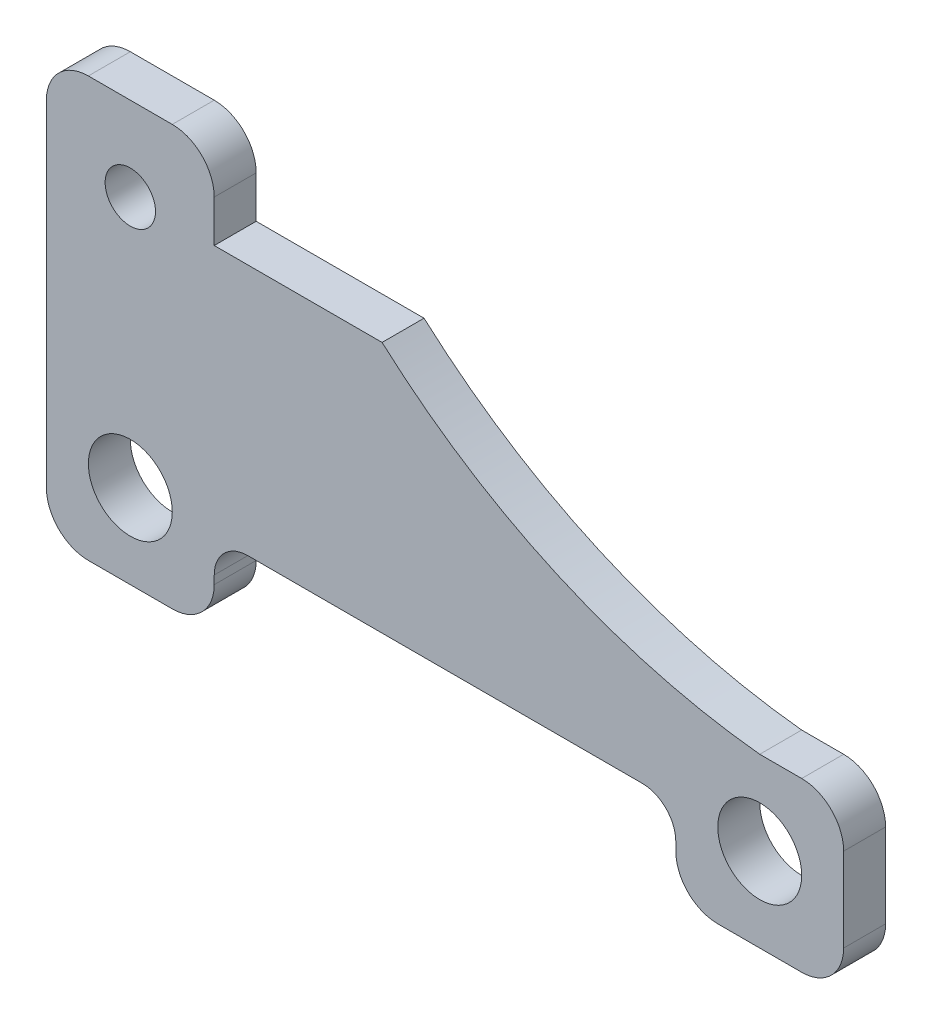
SolidWorks part; units mm, degrees
material "Plain Carbon Steel"
ref_plane "Front Plane" through (0, 0, 0) normal (0, 0, 1) x (1, 0, 0)
ref_plane "Top Plane" through (0, 0, 0) normal (0, 1, 0) x (1, 0, 0)
ref_plane "Right Plane" through (0, 0, 0) normal (1, 0, 0) x (0, 0, -1)
sketch "Carriage Plate Profile" plane through (0, 0, 0) normal (0, 0, 1) x (1, 0, 0)
  line L0 (-10, -5) -> (-10, 35)
  line L1 (-5, 40) -> (5, 40)
  line L2 (-5, -10) -> (5, -10)
  line L3 (10, -5) -> (10, -4)
  line L4 (14, 0) -> (61, 0)
  line L5 (65, -4) -> (65, -5)
  line L6 (70, -10) -> (75, -10)
  line L7 (10, 35) -> (10, 30)
  line L8 (75, -10) -> (80, -10)
  line L9 (85, -5) -> (85, 5)
  line L10 (80, 10) -> (75, 10)
  line L11 (10, 30) -> (30, 30)
  circle A0 centre (0, 0) radius 5
  circle A1 centre (75, 0) radius 5
  circle A2 centre (0, 30) radius 3
  arc A3 (85, 5) -> (80, 10) centre (80, 5) ccw
  arc A4 (5, 40) -> (10, 35) centre (5, 35) cw
  arc A5 (-10, 35) -> (-5, 40) centre (-5, 35) cw
  arc A6 (-10, -5) -> (-5, -10) centre (-5, -5) ccw
  arc A7 (5, -10) -> (10, -5) centre (5, -5) ccw
  arc A8 (65, -5) -> (70, -10) centre (70, -5) ccw
  arc A9 (80, -10) -> (85, -5) centre (80, -5) ccw
  arc A10 (10, -4) -> (14, 0) centre (14, -4) cw
  arc A11 (61, 0) -> (65, -4) centre (61, -4) cw
  arc A12 (75, 10) -> (30, 30) centre (83.4139, 89.5563) cw
  dimension "D1" = 5
  dimension "D2" = 4
  dimension "D3" = 10
  dimension "D4" = 6
  dimension "D6" = 30
  dimension "D7" = 10
  dimension "D9" = 5
  dimension "D20" = 80
  dimension "D5" = 50
  dimension "D8" = 75
  dimension "D10" = 5
  dimension "D11" = 5
  dimension "D12" = 5
  dimension "D13" = 5
  dimension "D14" = 5
  dimension "D15" = 5
  dimension "D16" = 5
  dimension "D17" = 20
  dimension "D18" = 30
  dimension "D19" = 10
extrude "Carriage Plate 5mm" add sketch "Carriage Plate Profile" along normal blind 5
